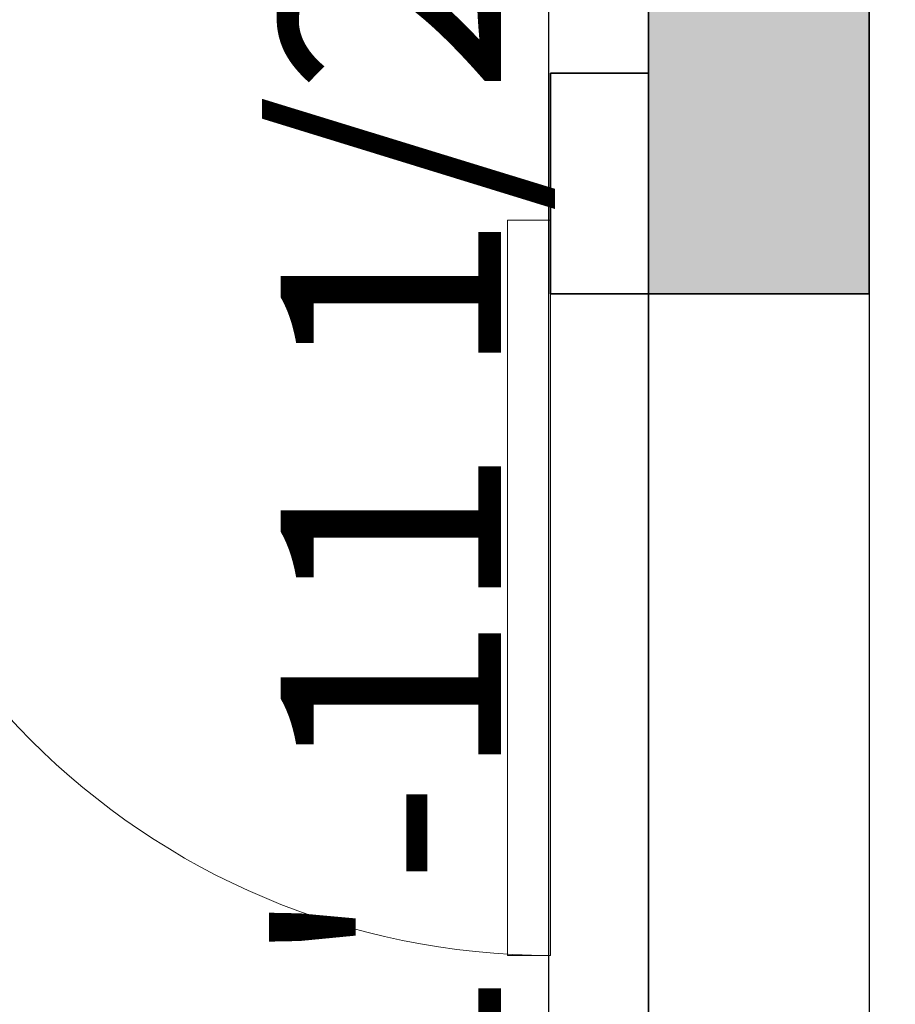
# Model space of a CAD drawing. Units: inches. Extents: x 3321 to 5237, y 11 to 1752.
# Tile 34 of 43: x 5095 to 5131, y 1396 to 1437. Entities that reach past the tile are written whole.
import ezdxf

# ---------------------------------------------------------------- set-up
doc = ezdxf.new("R2010")
doc.units = ezdxf.units.IN
for name, color, linetype, lineweight in [('A-ANNO-DIMS', 2, 'Continuous', 18), ('A-COLS', 1, 'Continuous', 35), ('A-DOOR', 4, 'Continuous', 18), ('A-FLOR-EDGE', 7, 'Continuous', 25), ('A-WALL', 7, 'Continuous', 35)]:
    doc.layers.add(name, color=color, linetype=linetype, lineweight=lineweight)
doc.styles.get("Standard").update_dxf_attribs({"font": 'arial.ttf'})
doc.dimstyles.new('ISO-25', dxfattribs={"dimtxt": 9, "dimasz": 2.5, "dimexe": 1.25, "dimexo": 0.625, "dimtad": 1, "dimdec": 1, "dimlunit": 3, "dimtxsty": 'Standard', "dimcen": 2.5, "dimclrd": 4, "dimclre": 4, "dimclrt": 256, "dimadec": 0, "dimazin": 0, "dimtfac": 1, "dimtdec": 1, "dimtmove": 0, "dimatfit": 3, "dimfxl": 1, "dimarcsym": 0})

# ---------------------------------------------------------------- blocks, each defined once
blk = doc.blocks.new('*U8')
for p, q in [((-30, 0), (-30, 6)), ((0, 0), (0, 6))]:
    blk.add_line(p, q)
blk.add_lwpolyline([(0, 0), (0, -30), (-1.75, -30), (-1.75, 0)], close=True)
blk.add_arc((0, 0), 30, 180, 270)
blk = doc.blocks.new('COL-9X12-FURN-PLAN')
h = blk.add_hatch(color=256)
h.dxf.hatch_style = 1
h.paths.add_polyline_path([(0, 12), (0, 0), (9, 0), (9, 12)])
blk.add_lwpolyline([(0, 0), (9, 0), (9, 12), (0, 12)], close=True)
blk = doc.blocks.new('*D194')
at = {"layer": 'A-ANNO-DIMS', "color": 4, "lineweight": -2, "transparency": 16777216}
for p, q in [((5037.321, 1452.516), (5037.321, 1436.712)), ((5121.084, 1452.516), (5121.084, 1436.712)), ((5039.821, 1437.962), (5118.584, 1437.962))]:
    blk.add_line(p, q, dxfattribs=at)
at = {"layer": 'A-ANNO-DIMS', "color": 4, "transparency": 16777216}
for points in [[(5039.821, 1438.379), (5039.821, 1437.545), (5037.321, 1437.962)], [(5118.584, 1438.379), (5118.584, 1437.545), (5121.084, 1437.962)]]:
    blk.add_solid(points, dxfattribs=at)
at = {"layer": 'Defpoints', "color": 0, "transparency": 16777216}
for p in [(5037.321, 1453.141), (5121.084, 1453.141), (5121.084, 1437.962)]:
    blk.add_point(p, dxfattribs=at)
at = {"layer": 'A-ANNO-DIMS', "transparency": 16777216, "insert": (5079.203, 1443.182), "char_height": 9, "attachment_point": 5}
blk.add_mtext('7\'-0" TYP.', dxfattribs=at)
blk = doc.blocks.new('*D197')
at = {"layer": 'A-ANNO-DIMS', "color": 4, "lineweight": -2, "transparency": 16777216}
for p, q in [((5117.009, 1364.83), (5117.009, 1476.212)), ((5114.11, 1364.83), (5118.259, 1364.83)), ((5117.009, 1343.839), (5117.009, 1362.33)), ((5114.11, 1341.339), (5118.259, 1341.339))]:
    blk.add_line(p, q, dxfattribs=at)
at = {"layer": 'A-ANNO-DIMS', "color": 4, "transparency": 16777216}
for points in [[(5116.592, 1362.33), (5117.426, 1362.33), (5117.009, 1364.83)], [(5116.592, 1343.839), (5117.426, 1343.839), (5117.009, 1341.339)]]:
    blk.add_solid(points, dxfattribs=at)
at = {"layer": 'Defpoints', "color": 0, "transparency": 16777216}
for p in [(5113.485, 1364.83), (5117.009, 1364.83), (5113.485, 1341.339)]:
    blk.add_point(p, dxfattribs=at)
at = {"layer": 'A-ANNO-DIMS', "transparency": 16777216, "insert": (5111.731, 1421.771), "char_height": 9, "attachment_point": 5, "rotation": 90}
blk.add_mtext('WC 1\'-11 1/2" TYP.', dxfattribs=at)

msp = doc.modelspace()

# ---------------------------------------------------------------- linework, layer by layer
at = {"layer": 'A-FLOR-EDGE'}
msp.add_line((5130.084, 1687.339), (5130.084, 1091.339), dxfattribs=at)
at = {"layer": 'A-WALL'}
for p, q in [((5121.084, 1554.339), (5121.084, 1434.339)), ((5117.084, 1434.339), (5117.084, 1425.339)), ((5117.084, 1434.339), (5121.084, 1434.339)), ((5117.084, 1425.339), (5121.084, 1425.339)), ((5121.084, 1425.339), (5121.084, 1341.339))]:
    msp.add_line(p, q, dxfattribs=at)

# ---------------------------------------------------------------- block references
at = {"layer": 'A-COLS'}
msp.add_blockref('COL-9X12-FURN-PLAN', (5121.084, 1425.339), dxfattribs=at)
at = {"layer": 'A-DOOR'}
msp.add_blockref('*U8', (5117.084, 1428.339), dxfattribs=at)

# ---------------------------------------------------------------- dimensions: what is measured, and where the dimension line sits
at = {"layer": 'A-ANNO-DIMS'}
dim = msp.add_linear_dim(base=(5117.009, 1364.83), p1=(5113.485, 1341.339), p2=(5113.485, 1364.83), angle=90, text='WC <> TYP.', dimstyle='ISO-25', override={"dimdec": 1, "dimlfac": 1, "dimrnd": 0, "dimzin": 1, "dimdsep": 46, "dimlunit": 4, "dimfrac": 2}, dxfattribs=at)
dim.commit()
dim.dimension.update_dxf_attribs({"geometry": '*D197', "text_midpoint": (5111.731, 1421.771)})
dim = msp.add_linear_dim(base=(5121.084, 1437.962), p1=(5037.321, 1453.141), p2=(5121.084, 1453.141), text='<> TYP.', dimstyle='ISO-25', override={"dimdec": 1, "dimlfac": 1, "dimrnd": 0, "dimzin": 1, "dimdsep": 46, "dimlunit": 4, "dimfrac": 2}, dxfattribs=at)
dim.commit()
dim.dimension.update_dxf_attribs({"geometry": '*D194', "text_midpoint": (5079.203, 1443.182)})

doc.saveas('drawing.dxf')
